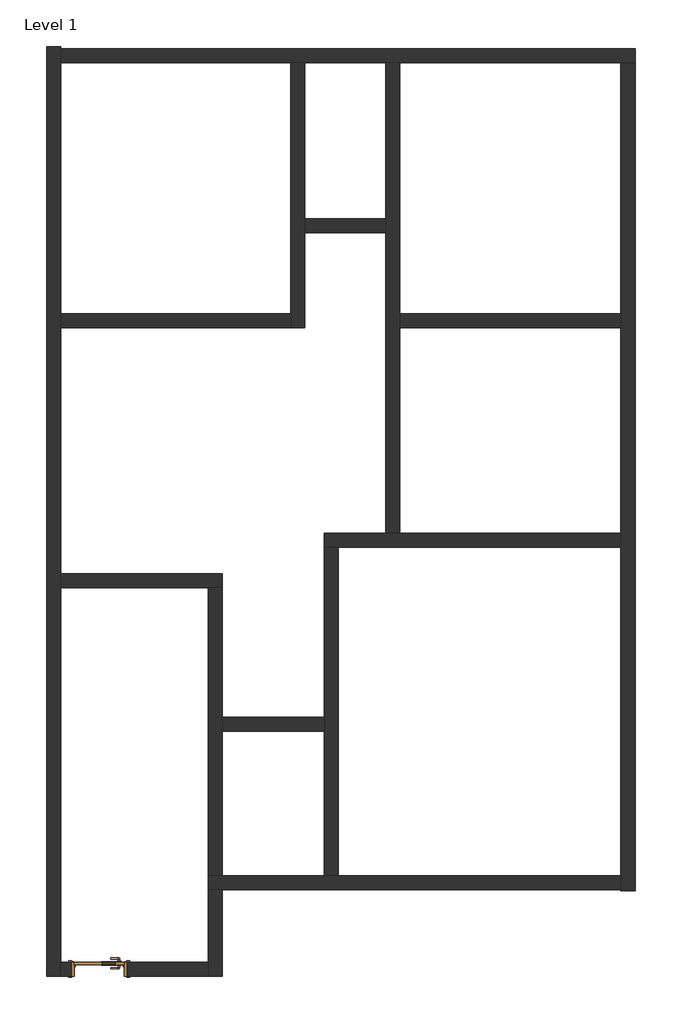
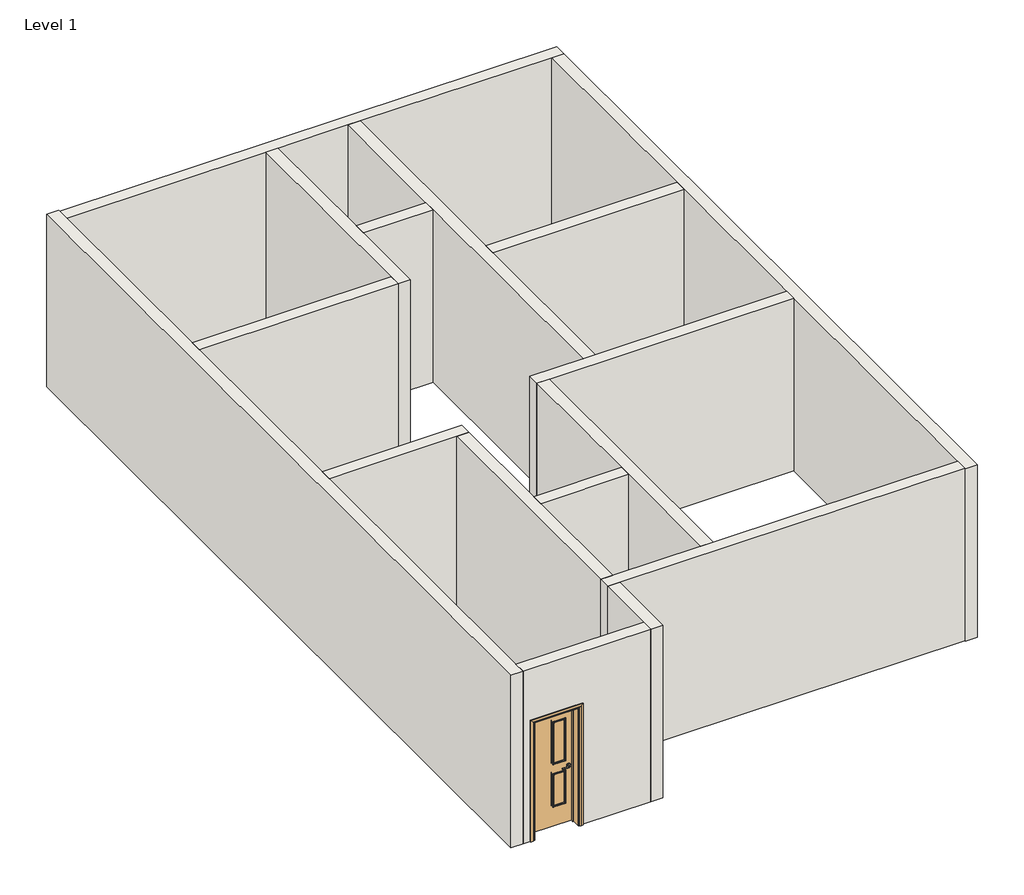
# One storey: 16 walls, 1 door.
"""IFC4 building model written with IfcOpenShell, lengths in millimetres."""

from ifc_helpers import new_model, si_unit, frame, origin, origin_with_axes, place, context, project, spatial, polyline, outline, extrude, faceted_brep, transform, mapped, element, save
from components import doors_intsgl_3_810x2110_fc3e9706

model = new_model("IFC4")

# Units and contexts
model_context = context("Model", 3, world=origin())
ifc_project = project(units=[si_unit("LENGTHUNIT", "METRE", prefix="MILLI")], contexts=[model_context])

# Site, building, storey
site = spatial("IfcSite", under=ifc_project)
building = spatial("IfcBuilding", under=site)
storey = spatial("IfcBuildingStorey", under=building, Name="Level 1", Elevation=0.0)

# Door
placement = place(None, origin())
doors_intsgl_3_810x2110_shape = doors_intsgl_3_810x2110_fc3e9706(model_context)
element("IfcDoor", 1, ObjectType="Doors_IntSgl_3 : 810x2110", at=placement, inside=storey, context=model_context, shape_type="MappedRepresentation", body=[
    mapped(doors_intsgl_3_810x2110_shape, transform((2047.129247, 10666.9898222, 0.0), x_axis=(-1.0, 0.0, 0.0), y_axis=(0.0, -1.0, 0.0), z_axis=(0.0, 0.0, 1.0))),
])

# Walls
element("IfcWall", 2, ObjectType="4.5\" p", at=placement, inside=storey, context=model_context, shape_type="Brep", body=[
    faceted_brep([(4815.729247, 23773.3898222, 0.0), (4815.729247, 20141.1898222, 0.0), (4815.729247, 19937.9898222, 0.0), (4815.729247, 19937.9898222, 3048.0), (4815.729247, 20141.1898222, 3048.0), (4815.729247, 23773.3898222, 3048.0), (5018.929247, 23773.3898222, 0.0), (5018.929247, 23773.3898222, 3048.0), (5018.929247, 21512.7898222, 3048.0), (5018.929247, 21309.5898222, 3048.0), (5018.929247, 19937.9898222, 3048.0), (5018.929247, 19937.9898222, 0.0), (5018.929247, 21309.5898222, 0.0), (5018.929247, 21512.7898222, 0.0)], [[[0, 1, 2, 3, 4, 5]], [[6, 7, 8, 9, 10, 11, 12, 13]], [[2, 1, 0, 6, 13, 12, 11]], [[5, 4, 3, 10, 9, 8, 7]], [[0, 5, 7, 6]], [[3, 2, 11, 10]]]),
])
element("IfcWall", 3, ObjectType="4.5\" p", at=placement, inside=storey, context=model_context, shape_type="SweptSolid", body=[
    extrude(outline(polyline([(4815.729247, 19937.9898222), (1488.329247, 19937.9898222), (1488.329247, 20141.1898222), (4815.729247, 20141.1898222), (4815.729247, 19937.9898222)])), origin_with_axes(), (0.0, 0.0, 1.0), 3048.0),
])
element("IfcWall", 4, ObjectType="4.5\" p", at=placement, inside=storey, context=model_context, shape_type="Brep", body=[
    faceted_brep([(6187.329247, 23773.3898222, 0.0), (6187.329247, 21512.7898222, 0.0), (6187.329247, 21309.5898222, 0.0), (6187.329247, 16966.1898222, 0.0), (6187.329247, 16966.1898222, 3048.0), (6187.329247, 21309.5898222, 3048.0), (6187.329247, 21512.7898222, 3048.0), (6187.329247, 23773.3898222, 3048.0), (6390.529247, 23773.3898222, 0.0), (6390.529247, 23773.3898222, 3048.0), (6390.529247, 20141.1898222, 3048.0), (6390.529247, 19937.9898222, 3048.0), (6390.529247, 16966.1898222, 3048.0), (6390.529247, 16966.1898222, 0.0), (6390.529247, 19937.9898222, 0.0), (6390.529247, 20141.1898222, 0.0)], [[[0, 1, 2, 3, 4, 5, 6, 7]], [[8, 9, 10, 11, 12, 13, 14, 15]], [[3, 2, 1, 0, 8, 15, 14, 13]], [[7, 6, 5, 4, 12, 11, 10, 9]], [[0, 7, 9, 8]], [[4, 3, 13, 12]]]),
])
element("IfcWall", 5, ObjectType="4.5\" p", at=placement, inside=storey, context=model_context, shape_type="SweptSolid", body=[
    extrude(outline(polyline([(6187.329247, 21309.5898222), (5018.929247, 21309.5898222), (5018.929247, 21512.7898222), (6187.329247, 21512.7898222), (6187.329247, 21309.5898222)])), origin_with_axes(), (0.0, 0.0, 1.0), 3048.0),
])
element("IfcWall", 6, ObjectType="4.5\" p", at=placement, inside=storey, context=model_context, shape_type="SweptSolid", body=[
    extrude(outline(polyline([(9590.929247, 19937.9898222), (6390.529247, 19937.9898222), (6390.529247, 20141.1898222), (9590.929247, 20141.1898222), (9590.929247, 19937.9898222)])), origin_with_axes(), (0.0, 0.0, 1.0), 3048.0),
])
element("IfcWall", 7, ObjectType="4.5\" p", at=placement, inside=storey, context=model_context, shape_type="Brep", body=[
    faceted_brep([(9590.929247, 16966.1898222, 0.0), (6390.529247, 16966.1898222, 0.0), (6187.329247, 16966.1898222, 0.0), (5298.329247, 16966.1898222, 0.0), (5298.329247, 16966.1898222, 3048.0), (6187.329247, 16966.1898222, 3048.0), (6390.529247, 16966.1898222, 3048.0), (9590.929247, 16966.1898222, 3048.0), (9590.929247, 16762.9898222, 0.0), (9590.929247, 16762.9898222, 3048.0), (5501.529247, 16762.9898222, 3048.0), (5298.329247, 16762.9898222, 3048.0), (5298.329247, 16762.9898222, 0.0), (5501.529247, 16762.9898222, 0.0)], [[[0, 1, 2, 3, 4, 5, 6, 7]], [[8, 9, 10, 11, 12, 13]], [[3, 2, 1, 0, 8, 13, 12]], [[7, 6, 5, 4, 11, 10, 9]], [[0, 7, 9, 8]], [[4, 3, 12, 11]]]),
])
element("IfcWall", 8, ObjectType="4.5\" p", at=placement, inside=storey, context=model_context, shape_type="Brep", body=[
    faceted_brep([(5298.329247, 16762.9898222, 0.0), (5298.329247, 14308.4690676, 0.0), (5298.329247, 14105.2690676, 0.0), (5298.329247, 12013.1898222, 0.0), (5298.329247, 12013.1898222, 3048.0), (5298.329247, 14105.2690676, 3048.0), (5298.329247, 14308.4690676, 3048.0), (5298.329247, 16762.9898222, 3048.0), (5501.529247, 16762.9898222, 0.0), (5501.529247, 16762.9898222, 3048.0), (5501.529247, 12013.1898222, 3048.0), (5501.529247, 12013.1898222, 0.0)], [[[0, 1, 2, 3, 4, 5, 6, 7]], [[8, 9, 10, 11]], [[3, 2, 1, 0, 8, 11]], [[7, 6, 5, 4, 10, 9]], [[0, 7, 9, 8]], [[4, 3, 11, 10]]]),
])
element("IfcWall", 9, ObjectType="4.5\" p", at=placement, inside=storey, context=model_context, shape_type="SweptSolid", body=[
    extrude(outline(polyline([(5298.329247, 14105.2690676), (3825.129247, 14105.2690676), (3825.129247, 14308.4690676), (5298.329247, 14308.4690676), (5298.329247, 14105.2690676)])), origin_with_axes(), (0.0, 0.0, 1.0), 3048.0),
])
element("IfcWall", 10, ObjectType="4.5\" p", at=placement, inside=storey, context=model_context, shape_type="Brep", body=[
    faceted_brep([(1488.329247, 16178.7898222, 0.0), (3621.929247, 16178.7898222, 0.0), (3825.129247, 16178.7898222, 0.0), (3825.129247, 16178.7898222, 3048.0), (3621.929247, 16178.7898222, 3048.0), (1488.329247, 16178.7898222, 3048.0), (1488.329247, 16381.9898222, 0.0), (1488.329247, 16381.9898222, 3048.0), (3825.129247, 16381.9898222, 3048.0), (3825.129247, 16381.9898222, 0.0)], [[[0, 1, 2, 3, 4, 5]], [[6, 7, 8, 9]], [[2, 1, 0, 6, 9]], [[5, 4, 3, 8, 7]], [[0, 5, 7, 6]], [[3, 2, 9, 8]]]),
])
element("IfcWall", 11, ObjectType="4.5\" p", at=placement, inside=storey, context=model_context, shape_type="Brep", body=[
    faceted_brep([(3621.929247, 16178.7898222, 0.0), (3621.929247, 12013.1898222, 0.0), (3621.929247, 12013.1898222, 3048.0), (3621.929247, 16178.7898222, 3048.0), (3825.129247, 16178.7898222, 0.0), (3825.129247, 16178.7898222, 3048.0), (3825.129247, 14308.4690676, 3048.0), (3825.129247, 14105.2690676, 3048.0), (3825.129247, 12013.1898222, 3048.0), (3825.129247, 12013.1898222, 0.0), (3825.129247, 14105.2690676, 0.0), (3825.129247, 14308.4690676, 0.0)], [[[0, 1, 2, 3]], [[4, 5, 6, 7, 8, 9, 10, 11]], [[1, 0, 4, 11, 10, 9]], [[3, 2, 8, 7, 6, 5]], [[2, 1, 9, 8]], [[0, 3, 5, 4]]]),
])
element("IfcWall", 12, ObjectType="4.5\" p", at=placement, inside=storey, context=model_context, shape_type="SweptSolid", body=[
    extrude(outline(polyline([(3048.0, 3621.929247), (3048.0, 1488.329247), (0.0, 1488.329247), (0.0, 1642.129247), (2110.0, 1642.129247), (2110.0, 2452.129247), (0.0, 2452.129247), (0.0, 3621.929247), (3048.0, 3621.929247)])), frame((0.0, 10565.3898222, 0.0), z_axis=(0.0, 1.0, 0.0), x_axis=(0.0, 0.0, 1.0)), (0.0, 0.0, 1.0), 203.2),
])
element("IfcWall", 13, ObjectType="9\"", at=placement, inside=storey, context=model_context, shape_type="Brep", body=[
    faceted_brep([(1285.129247, 24005.1648222, 0.0), (1285.129247, 10565.3898222, 0.0), (1285.129247, 10565.3898222, 3048.0), (1285.129247, 24005.1648222, 3048.0), (1488.329247, 24005.1648222, 0.0), (1488.329247, 24005.1648222, 3048.0), (1488.329247, 23976.5898222, 3048.0), (1488.329247, 23773.3898222, 3048.0), (1488.329247, 20141.1898222, 3048.0), (1488.329247, 19937.9898222, 3048.0), (1488.329247, 16381.9898222, 3048.0), (1488.329247, 16178.7898222, 3048.0), (1488.329247, 10768.5898222, 3048.0), (1488.329247, 10565.3898222, 3048.0), (1488.329247, 10565.3898222, 0.0), (1488.329247, 10768.5898222, 0.0), (1488.329247, 16178.7898222, 0.0), (1488.329247, 16381.9898222, 0.0), (1488.329247, 19937.9898222, 0.0), (1488.329247, 20141.1898222, 0.0), (1488.329247, 23773.3898222, 0.0), (1488.329247, 23976.5898222, 0.0)], [[[0, 1, 2, 3]], [[4, 5, 6, 7, 8, 9, 10, 11, 12, 13, 14, 15, 16, 17, 18, 19, 20, 21]], [[1, 0, 4, 21, 20, 19, 18, 17, 16, 15, 14]], [[3, 2, 13, 12, 11, 10, 9, 8, 7, 6, 5]], [[0, 3, 5, 4]], [[2, 1, 14, 13]]]),
])
element("IfcWall", 14, ObjectType="9\"", at=placement, inside=storey, context=model_context, shape_type="Brep", body=[
    faceted_brep([(1488.329247, 23773.3898222, 0.0), (4815.729247, 23773.3898222, 0.0), (5018.929247, 23773.3898222, 0.0), (6187.329247, 23773.3898222, 0.0), (6390.529247, 23773.3898222, 0.0), (9590.929247, 23773.3898222, 0.0), (9794.129247, 23773.3898222, 0.0), (9794.129247, 23773.3898222, 3048.0), (9590.929247, 23773.3898222, 3048.0), (6390.529247, 23773.3898222, 3048.0), (6187.329247, 23773.3898222, 3048.0), (5018.929247, 23773.3898222, 3048.0), (4815.729247, 23773.3898222, 3048.0), (1488.329247, 23773.3898222, 3048.0), (1488.329247, 23976.5898222, 0.0), (1488.329247, 23976.5898222, 3048.0), (9794.129247, 23976.5898222, 3048.0), (9794.129247, 23976.5898222, 0.0)], [[[0, 1, 2, 3, 4, 5, 6, 7, 8, 9, 10, 11, 12, 13]], [[14, 15, 16, 17]], [[6, 5, 4, 3, 2, 1, 0, 14, 17]], [[13, 12, 11, 10, 9, 8, 7, 16, 15]], [[0, 13, 15, 14]], [[7, 6, 17, 16]]]),
])
element("IfcWall", 15, ObjectType="9\"", at=placement, inside=storey, context=model_context, shape_type="Brep", body=[
    faceted_brep([(9590.929247, 23773.3898222, 0.0), (9590.929247, 20141.1898222, 0.0), (9590.929247, 19937.9898222, 0.0), (9590.929247, 16966.1898222, 0.0), (9590.929247, 16762.9898222, 0.0), (9590.929247, 12013.1898222, 0.0), (9590.929247, 11809.9898222, 0.0), (9590.929247, 11797.2898222, 0.0), (9590.929247, 11797.2898222, 3048.0), (9590.929247, 11809.9898222, 3048.0), (9590.929247, 12013.1898222, 3048.0), (9590.929247, 16762.9898222, 3048.0), (9590.929247, 16966.1898222, 3048.0), (9590.929247, 19937.9898222, 3048.0), (9590.929247, 20141.1898222, 3048.0), (9590.929247, 23773.3898222, 3048.0), (9794.129247, 23773.3898222, 0.0), (9794.129247, 23773.3898222, 3048.0), (9794.129247, 11797.2898222, 3048.0), (9794.129247, 11797.2898222, 0.0)], [[[0, 1, 2, 3, 4, 5, 6, 7, 8, 9, 10, 11, 12, 13, 14, 15]], [[16, 17, 18, 19]], [[7, 6, 5, 4, 3, 2, 1, 0, 16, 19]], [[8, 7, 19, 18]], [[15, 14, 13, 12, 11, 10, 9, 8, 18, 17]], [[0, 15, 17, 16]]]),
])
element("IfcWall", 16, ObjectType="9\"", at=placement, inside=storey, context=model_context, shape_type="Brep", body=[
    faceted_brep([(9590.929247, 12013.1898222, 0.0), (5501.529247, 12013.1898222, 0.0), (5298.329247, 12013.1898222, 0.0), (3825.129247, 12013.1898222, 0.0), (3621.929247, 12013.1898222, 0.0), (3621.929247, 12013.1898222, 3048.0), (3825.129247, 12013.1898222, 3048.0), (5298.329247, 12013.1898222, 3048.0), (5501.529247, 12013.1898222, 3048.0), (9590.929247, 12013.1898222, 3048.0), (9590.929247, 11809.9898222, 0.0), (9590.929247, 11809.9898222, 3048.0), (3825.129247, 11809.9898222, 3048.0), (3621.929247, 11809.9898222, 3048.0), (3621.929247, 11809.9898222, 0.0), (3825.129247, 11809.9898222, 0.0)], [[[0, 1, 2, 3, 4, 5, 6, 7, 8, 9]], [[10, 11, 12, 13, 14, 15]], [[4, 3, 2, 1, 0, 10, 15, 14]], [[9, 8, 7, 6, 5, 13, 12, 11]], [[0, 9, 11, 10]], [[5, 4, 14, 13]]]),
])
element("IfcWall", 17, ObjectType="9\"", at=placement, inside=storey, context=model_context, shape_type="Brep", body=[
    faceted_brep([(3621.929247, 11809.9898222, 0.0), (3621.929247, 10768.5898222, 0.0), (3621.929247, 10565.3898222, 0.0), (3621.929247, 10565.3898222, 3048.0), (3621.929247, 10768.5898222, 3048.0), (3621.929247, 11809.9898222, 3048.0), (3825.129247, 11809.9898222, 0.0), (3825.129247, 11809.9898222, 3048.0), (3825.129247, 10565.3898222, 3048.0), (3825.129247, 10565.3898222, 0.0)], [[[0, 1, 2, 3, 4, 5]], [[6, 7, 8, 9]], [[2, 1, 0, 6, 9]], [[5, 4, 3, 8, 7]], [[0, 5, 7, 6]], [[3, 2, 9, 8]]]),
])

save(model, "model.ifc")

# Revit data of these elements
# Type "Doors_IntSgl_3 : 810x2110"
#   Type Mark = "11"
#   Type Comments = "Internal Single"
#   Operation = "SingleSwingRight"
#   Construction Type Id = "SGL"
#   Manufacturer = "Revit"
#   Keynote = "L20"
#   Description = "Internal Single Door"
#   Analytic Construction = "Large single-glazed windows"
#   Visual Light Transmittance = 0.9
#   VisionPanel Width = 0' - 7.87402"
#   UnderCut = 0' - 0.31496"
#   Tolerance = 0' - 0.07874"
#   Structural Tolerance = 0' - 0.31496"
#   StopDepth = 0' - 1.25984"
#   Stop Thickness = 0' - 0.74803"
#   Stile Top of Lock Rail = 3' - 7.30709"
#   Stile Top Rail = 0' - 8.85827"
#   Stile Shutting = 0' - 4.92126"
#   Stile Lock Rail = 0' - 6.88976"
#   Stile Bottom Rail = 1' - 1.77953"
#   Solar Heat Gain Coefficient = 0.86
#   Rough Width = 2' - 7.88976"
#   Rough Height = 6' - 11.07087"
#   Heat Transfer Coefficient (U) = 0.979472 BTU/(h·ft²·°F)
#   Handle Z Distance = 3' - 3.37008"
#   Handle X Distance = 0' - 2.95276"
#   Frame Thickness = 0' - 1.25984"
#   Door Panel Width = 2' - 4.58268"
#   Door Panel Thickness = 0' - 1.49606"
#   Door Panel Offset = 0' - 0"
#   Height = 6' - 11.07087"
#   Width = 2' - 7.88976"
#   Door Panel Height = 6' - 9.10236"
#   Architrave Setback = 0' - 0.19685"
#   Vis - Ironmongery = yes
#   Define Thermal Properties by = 1
#   Material Ironmongery = Door - Handle
#   Material Glass = Door - Glazing
#   Material Frame = Door - Frame/Mullion
#   Material Door = Door - Panel
#   Material Beading = Door - Panel
#   Material Architrave = Door - Architrave
#   Function = (empty or 0)
#   Wall Closure = (empty or 0)
# Type "4.5\" p"
#   Assembly Code = "B2010"
#   Layers, outside or top first: 0' - 8" no material (function 1)
# Type "9\""
#   Assembly Code = "B2010"
#   Layers, outside or top first: 0' - 8" no material (function 1)
# Element 1 (IfcDoor, "Doors_IntSgl_3 : 810x2110")
#   Phase Created = New Construction
#   Materials on its faces: "Door - Panel", "Door - Architrave", "Door - Handle", "Door - Frame/Mullion", "Door - Glazing"
# Elements 2, 3, 4, 5, 6, 7, 8, 9, 10, 11, 12 (IfcWall, "4.5\" p")
#   Top Offset = 0' - 0"
#   Base Offset = 0' - 0"
#   wall height = 10' - 0"
#   Phase Created = New Construction
#   Base Constraint = Level 1
#   Top Constraint = Level 2
#   Materials on its faces: "Default Wall"
# Elements 13, 14, 15, 16, 17 (IfcWall, "9\"")
#   Top Offset = 0' - 0"
#   Base Offset = 0' - 0"
#   wall height = 10' - 0"
#   Phase Created = New Construction
#   Base Constraint = Level 1
#   Top Constraint = Level 2
#   Materials on its faces: "Default Wall"
# Materials
#   "Door - Handle": colour RGB 247 247 247, transparency 0
#   "Door - Glazing": colour RGB 0 0 255, transparency 0.75
#   "Door - Frame/Mullion": class "Wood", colour RGB 212 179 113, transparency 0
#   "Door - Panel": class "Wood", colour RGB 210 159 95, transparency 0, Cost = 0
#   "Door - Architrave": class "Wood", colour RGB 212 179 113, transparency 0
#   "Default Wall": colour RGB 128 128 128, transparency 0, Cost = 0
